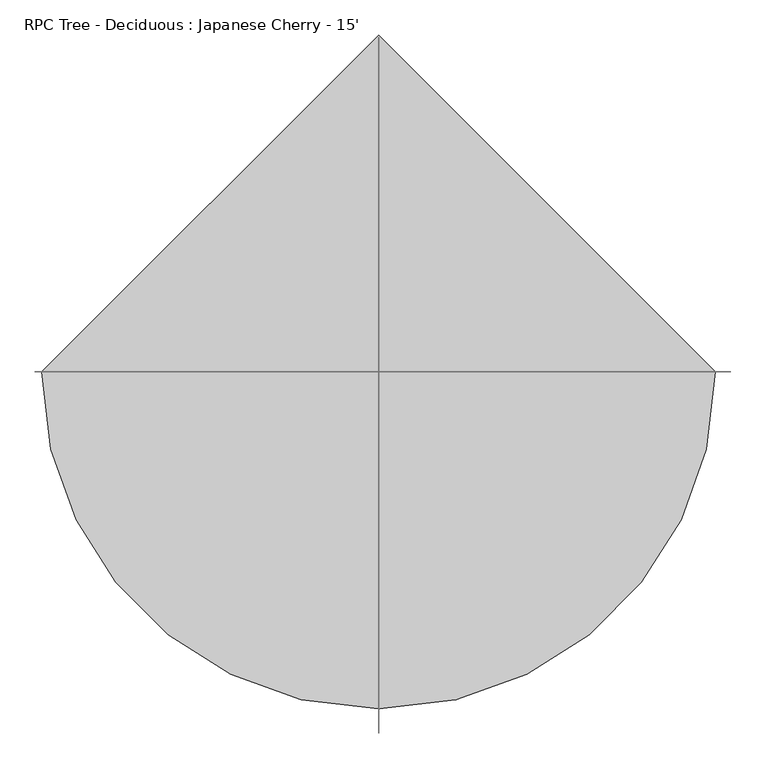
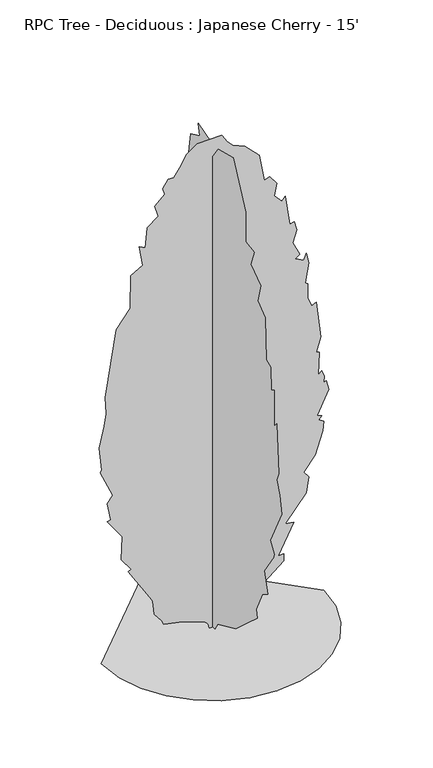
"""IFC4 building model written with IfcOpenShell, lengths in millimetres: geographic element geometry, RPC Tree - Deciduous : Japanese Cherry - 15'."""

from ifc_helpers import new_model, si_unit, origin, place, context, project, spatial, triangles, source, transform, mapped, element, save


def rpc_tree_deciduous_japanese_cherry_15_bc05297b(model_context):
    return source(origin(), model_context, "Body", "Tessellation", [
        triangles([(-31.5306812, 1.4e-06, 2.8e-06), (-39.0081023, -6e-07, 38.4422075), (-59.1836422, -1.3e-06, 65.1245405), (-265.2111374, 3.2e-06, 140.9481372), (-432.584424, 8.4e-06, 176.4639745), (-448.6267588, 6.7e-06, 216.5692663), (-513.2636201, 4.6e-06, 299.3118357), (-528.8383962, -2.2e-06, 425.1173653), (-552.9035334, -4e-06, 473.2437881), (-745.4071175, -1.38e-05, 778.0426254), (-720.5004982, -1.58e-05, 793.0104618), (-805.6760405, -1.92e-05, 912.4162548), (-797.0436459, -3.22e-05, 1124.2039816), (-929.893313, -3.73e-05, 1307.438364), (-897.8076262, -3.92e-05, 1315.4557526), (-928.6469501, -4.75e-05, 1477.5445507), (-881.7620213, -5.33e-05, 1540.0450962), (-994.0593819, -6.32e-05, 1788.7027382), (-978.0192272, -6.48e-05, 1804.7428928), (-1002.0822206, -7.67e-05, 2021.3094704), (-958.5500668, -8.98e-05, 2210.2588383), (-937.9107016, -9.72e-05, 2318.0930992), (-945.9334677, -0.0001059, 2470.4936806), (-849.681712, -0.000146, 3072.0726585), (-729.3669628, -0.0001608, 3232.496006), (-722.8627087, -0.0001789, 3531.9140671), (-617.0696022, -0.0001872, 3593.4457764), (-649.1552891, -0.0001968, 3777.9263763), (-594.3945691, -0.0001973, 3746.5102707), (-576.9664905, -0.000209, 3930.3269577), (-480.7108832, -0.0002176, 4002.5158653), (-512.7955164, -0.0002224, 4106.7903145), (-424.5632566, -0.000231, 4187.0019882), (-440.6055914, -0.0002337, 4243.1505959), (-392.4791685, -0.0002401, 4315.3395035), (-344.3527093, -0.0002422, 4315.3395035), (-289.1347498, -0.0002488, 4387.0330925), (-233.7763556, -0.0002575, 4491.1008682), (-134.4542386, -0.0002658, 4558.3583908), (79.1094609, -0.0002754, 4561.7166161), (128.8910789, -0.0002729, 4483.7800941), (177.0175199, -0.0002721, 4435.6542526), (284.0162759, -0.0002741, 4390.3369606), (409.6285578, -0.0002718, 4259.1908958), (457.755017, -0.0002591, 4010.5386314), (505.8814399, -0.0002621, 4026.5786407), (564.5784748, -0.0002597, 3942.6061501), (545.9856417, -0.0002524, 3834.0752747), (610.1570881, -0.0002509, 3761.886367), (642.2373974, -0.0002542, 3793.9719086), (682.3459957, -0.0002397, 3521.2513458), (722.4490711, -0.0002419, 3529.2741119), (744.2586411, -0.0002382, 3449.8135551), (708.4119192, -0.0002301, 3340.776606), (770.5749853, -0.0002249, 3208.4329399), (728.5450653, -0.0002216, 3183.2324432), (802.6607449, -0.0002225, 3144.2615662), (826.7236656, -0.0002269, 3200.4101738), (850.7865864, -0.0002222, 3104.1584908), (818.7062771, -0.0002103, 2927.695134), (841.8657646, -0.0002102, 2908.6396111), (838.6490278, -0.0002023, 2778.3478546), (874.8495798, -0.0001989, 2695.0828789), (914.9581055, -0.0002016, 2711.1228882), (955.0611809, -0.0001833, 2374.2417068), (914.9581055, -0.0001739, 2245.9041916), (939.9354326, -0.0001744, 2237.4188084), (930.9982601, -0.0001617, 2029.3322365), (963.0840197, -0.0001645, 2053.3951572), (987.1469404, -0.0001622, 1997.2465496), (979.1241743, -0.0001585, 1941.1031742), (1003.1870951, -0.00016, 1949.1205627), (1027.2500158, -0.0001558, 1860.8916458), (922.9754213, -0.0001388, 1652.3424568), (963.0840197, -0.0001396, 1636.3023022), (939.0210262, -0.0001367, 1604.21647), (979.1241743, -0.000137, 1580.1535492), (970.687698, -0.0001315, 1493.7044655), (906.9352667, -0.0001166, 1291.3926865), (802.6607449, -0.0001044, 1163.0551712), (850.7865864, -0.0001032, 1106.9064909), (824.4812153, -9.37e-05, 966.7851746), (642.2373974, -7.21e-05, 737.9394773), (714.4316826, -7.47e-05, 729.9167112), (578.0713649, -5.3e-05, 465.2226208), (626.1972427, -5.51e-05, 465.2226208), (626.1972427, -5.13e-05, 401.0538631), (273.269312, -1.86e-05, 112.2952078), (273.269312, -2.1e-05, 152.4004905), (32.6379787, -1.4e-06, 0.0), (2.3e-06, 29.5482237, 0.0002786), (5.5e-06, 73.888109, 30.635001), (1.1e-05, 165.906443, 64.1693117), (1.54e-05, 382.4757093, 144.3798682), (2.49e-05, 494.7708899, 248.6539176), (2.31e-05, 446.644467, 256.675085), (4.14e-05, 618.3105148, 504.1212276), (4.45e-05, 566.9624863, 625.6421167), (5.13e-05, 711.3401562, 834.1913057), (5.48e-05, 695.3000015, 930.4430614), (6.5e-05, 799.5691458, 1058.7806494), (7.32e-05, 834.6267443, 1212.2805822), (7.08e-05, 815.6147507, 1371.6043602), (8.48e-05, 943.9522659, 1564.108017), (9.35e-05, 951.9696545, 1756.6170513), (9.84e-05, 905.6399242, 1914.1555458), (0.0001039, 976.0325752, 2165.6925179), (0.0001049, 911.8665791, 2253.9215801), (0.0001126, 831.6549053, 2510.596756), (0.0001142, 887.8035856, 2687.0601128), (0.0001226, 823.6321392, 2943.7351433), (0.0001258, 743.4259157, 3096.1357246), (0.0001294, 703.3173901, 3416.9821289), (0.0001263, 655.1914759, 3392.9193535), (0.0001389, 655.1914759, 3681.6746933), (0.0001357, 558.9396838, 3705.7374687), (0.0001324, 508.0183007, 3877.0793358), (0.0001373, 478.7285914, 4018.5613976), (0.0001373, 382.4757093, 4114.8130806), (0.0001478, 334.3492501, 4403.5739433), (0.0001361, 197.9905493, 4467.7400848), (0.0001415, 218.699605, 4570.9913406), (0.0001303, 24.3187645, 4509.0241928), (0.0001324, 13.5058946, 4371.4881111), (0.0001255, -82.7469296, 4507.8486832), (0.0001182, -315.3579675, 4572.014534), (0.0001012, -507.8642767, 4178.9792221), (8.93e-05, -507.8642767, 3906.2638916), (8.27e-05, -634.726228, 3883.6815491), (7.88e-05, -580.0525666, 3737.8233009), (7.6e-05, -734.6628605, 3632.2806152), (7.05e-05, -692.3499636, 3465.1082611), (6.18e-05, -804.6419466, 3376.8738213), (5.28e-05, -820.6874788, 2991.8609848), (4.88e-05, -886.176214, 2963.9228645), (3.92e-05, -892.8763865, 2751.2314865), (3.85e-05, -941.002228, 2783.3117958), (3.23e-05, -941.002228, 2446.4306145), (2.41e-05, -981.1053761, 2494.556456), (1.17e-05, -1013.1911356, 2045.3777687), (9.8e-06, -978.3621569, 1968.9761822), (2.5e-06, -1029.2366678, 1852.8687344), (3.1e-06, -1053.2996613, 1692.4455322), (-4.6e-06, -884.8535477, 1347.5414394), (-1.13e-05, -941.002228, 1251.2896111), (-4e-06, -936.2560787, 1217.3097811), (-6.9e-06, -788.601792, 1002.6373466), (-1.74e-05, -844.7504723, 818.1511511), (-1.6e-05, -756.5160324, 762.0024708), (-1.2e-05, -668.2870428, 569.4988503), (-1.58e-05, -684.3271975, 497.3072903), (-1.51e-05, -523.9060664, 352.927949), (-1.44e-05, -355.4632593, 200.5274766), (-7.8e-06, -74.7246813, 72.1899341), (-5e-07, -34.6204386, 0.0002747), (-981.7802622, 0.0, 0.0003197), (-955.8231983, -224.9589068, 0.0003052), (-881.9035097, -431.5481137, 0.0002896), (-765.937623, -613.8474152, 0.0002737), (-613.8474152, -765.937623, 0.000258), (-431.5481137, -881.9035097, 0.0002431), (-224.9589068, -955.8231983, 0.0002297), (4.41e-05, -981.7802622, 0.0002183), (224.9589068, -955.8231983, 0.00021), (431.5481137, -881.9035097, 0.0002054), (613.8474152, -765.937623, 0.0002043), (765.937623, -613.8474152, 0.0002067), (881.9035097, -431.5475687, 0.0002125), (955.8231983, -224.9589068, 0.0002216), (981.7802622, 8.58e-05, 0.0002339), (-0.0001282, 981.7802622, 0.0003353)], [[57, 58, 59], [27, 28, 29], [87, 88, 89], [49, 50, 51], [13, 14, 15], [83, 84, 85], [74, 75, 76], [63, 64, 65], [68, 69, 70], [71, 72, 73], [9, 10, 11], [85, 86, 87], [85, 87, 89], [51, 52, 53], [54, 55, 56], [90, 1, 2], [66, 67, 68], [45, 46, 47], [17, 18, 19], [68, 70, 71], [45, 47, 48], [31, 32, 33], [76, 77, 78], [89, 90, 2], [89, 2, 3], [57, 59, 60], [51, 53, 54], [25, 26, 27], [39, 40, 41], [56, 57, 60], [71, 73, 74], [34, 35, 36], [33, 34, 36], [4, 5, 6], [60, 61, 62], [80, 81, 82], [38, 39, 41], [37, 38, 41], [37, 41, 42], [29, 30, 31], [15, 16, 17], [36, 37, 42], [33, 36, 42], [31, 33, 42], [31, 42, 43], [31, 43, 44], [31, 44, 45], [29, 31, 45], [29, 45, 48], [27, 29, 48], [25, 27, 48], [25, 48, 49], [25, 49, 51], [25, 51, 54], [25, 54, 56], [25, 56, 60], [25, 60, 62], [24, 25, 62], [23, 24, 62], [22, 23, 62], [22, 62, 63], [22, 63, 65], [22, 65, 66], [22, 66, 68], [21, 22, 68], [20, 21, 68], [19, 20, 68], [17, 19, 68], [17, 68, 71], [17, 71, 74], [15, 17, 74], [13, 15, 74], [13, 74, 76], [13, 76, 78], [13, 78, 79], [13, 79, 80], [12, 13, 80], [11, 12, 80], [9, 11, 80], [9, 80, 82], [9, 82, 83], [9, 83, 85], [9, 85, 89], [9, 89, 3], [9, 3, 4], [8, 9, 4], [8, 4, 6], [7, 8, 6], [138, 139, 140], [94, 95, 96], [136, 137, 138], [121, 122, 123], [112, 113, 114], [128, 129, 130], [121, 123, 124], [125, 126, 127], [124, 125, 127], [114, 115, 116], [147, 148, 149], [130, 131, 132], [124, 127, 128], [134, 135, 136], [154, 155, 91], [154, 91, 92], [150, 151, 152], [96, 97, 98], [119, 120, 121], [119, 121, 124], [119, 124, 128], [118, 119, 128], [117, 118, 128], [116, 117, 128], [116, 128, 130], [114, 116, 130], [114, 130, 132], [112, 114, 132], [112, 132, 133], [112, 133, 134], [112, 134, 136], [111, 112, 136], [110, 111, 136], [109, 110, 136], [109, 136, 138], [109, 138, 140], [109, 140, 141], [108, 109, 141], [107, 108, 141], [106, 107, 141], [105, 106, 141], [104, 105, 141], [103, 104, 141], [103, 141, 142], [103, 142, 143], [103, 143, 144], [102, 103, 144], [101, 102, 144], [100, 101, 144], [100, 144, 145], [100, 145, 146], [100, 146, 147], [100, 147, 149], [100, 149, 150], [100, 150, 152], [100, 152, 153], [100, 153, 154], [99, 100, 154], [98, 99, 154], [96, 98, 154], [96, 154, 92], [96, 92, 93], [96, 93, 94], [170, 171, 156], [169, 170, 156], [169, 156, 157], [168, 169, 157], [168, 157, 158], [168, 158, 159], [167, 168, 159], [166, 167, 159], [166, 159, 160], [166, 160, 161], [166, 161, 162], [166, 162, 163], [166, 163, 164], [166, 164, 165]], closed=False),
    ])


if __name__ == "__main__":
    model = new_model("IFC4")
    model_context = context("Model", 3, world=origin())
    ifc_project = project(units=[si_unit("LENGTHUNIT", "METRE", prefix="MILLI")], contexts=[model_context])
    site = spatial("IfcSite", under=ifc_project)
    building = spatial("IfcBuilding", under=site)
    placement = place(None, origin())
    rpc_tree_deciduous_japanese_cherry_15_shape = rpc_tree_deciduous_japanese_cherry_15_bc05297b(model_context)
    element("IfcGeographicElement", 1, ObjectType="RPC Tree - Deciduous : Japanese Cherry - 15'", at=placement, inside=building, context=model_context, shape_type="MappedRepresentation", body=[
        mapped(rpc_tree_deciduous_japanese_cherry_15_shape, transform((0.0, 0.0, 0.0), x_axis=(1.0, 0.0, 0.0), y_axis=(0.0, 1.0, 0.0), z_axis=(0.0, 0.0, 1.0))),
    ])
    save(model, "model.ifc")

# Revit data of these elements
# Type "RPC Tree - Deciduous : Japanese Cherry - 15'"
#   built-in parameter 1005195 = "RPC-16-FUM3-UUQ0-UBF0-N000-ST1L-LVER-AU"
#   Type Comments = "Japanese Cherry"
#   Assembly Code = "G2050500"
#   Height = 15' - 0"
#   Default Elevation = 0
